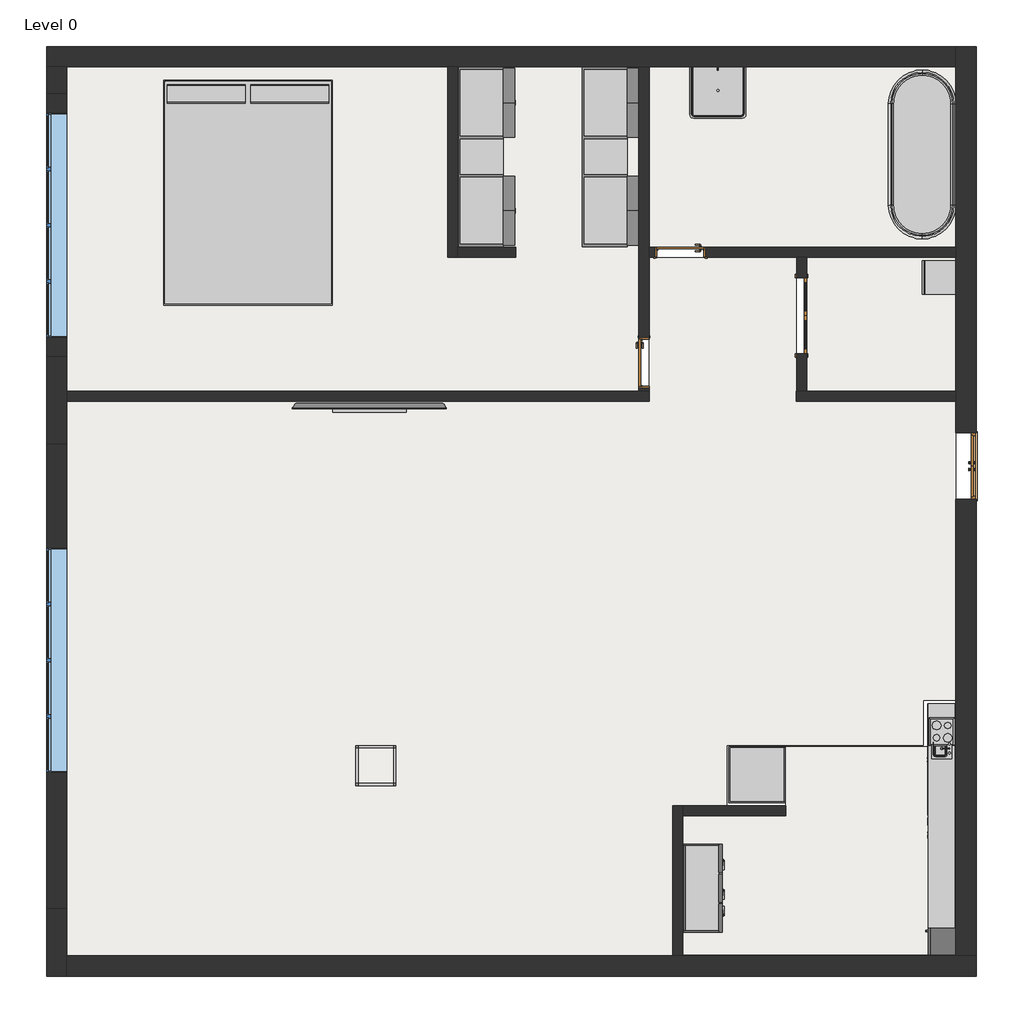
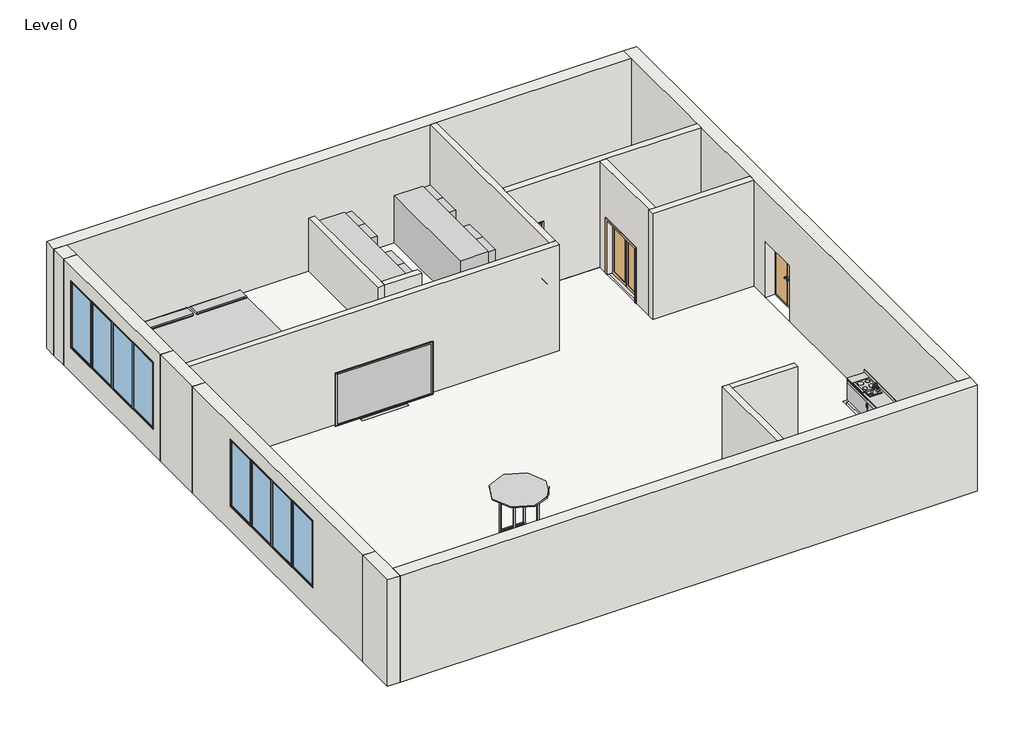
# One storey, incomplete: 17 walls, 7 furniture elements, 5 proxies, 4 doors, 4 flow terminals, 4 slabs, 2 windows.
"""IFC4 building model written with IfcOpenShell, lengths in millimetres."""

from ifc_helpers import new_model, si_unit, frame, origin, origin_with_axes, place, context, project, spatial, polyline, outline, extrude, faceted_brep, transform, mapped, element, save
from components import proxy_a6faaae8, proxy_45b28599, proxy_233f0198, kitchenette_medium_kitchenette_medium_eaec4ed0, proxy_c523a7b7, door_bbcd5f29, doors_extdbl_flush_1510x2110mm_ebd05307, doors_intsgl_1143x2413mm_ac4b68bc, flow_terminal_871c2e40, flow_terminal_6a24c7e0, flow_terminal_2cf38851, flow_terminal_2ef58978, furniture_0647d374, furniture_14b7b6c7, furniture_d6024f60, furniture_eacb8e26, furniture_d0237233, furniture_4371de90, window_3db9eff8

model = new_model("IFC4")

# Units and contexts
model_context = context("Model", 3, world=origin())
ifc_project = project(units=[si_unit("LENGTHUNIT", "METRE", prefix="MILLI")], contexts=[model_context])

# Site, building, storey
site = spatial("IfcSite", under=ifc_project)
building = spatial("IfcBuilding", under=site)
storey = spatial("IfcBuildingStorey", under=building, Name="Level 0", Elevation=0.0)

# Proxies
placement = place(None, origin())
proxy_shape = proxy_a6faaae8(model_context)
element("IfcBuildingElementProxy", 1, Name="Cook Top-4 Unit2 : 22\" x 20\"", ObjectType="Cook Top-4 Unit2 : 22\" x 20\"", at=placement, inside=storey, context=model_context, shape_type="MappedRepresentation", body=[
    mapped(proxy_shape, transform((-8192.0196087, -11110.3672005, 1.7), x_axis=(0.0, 1.0, 0.0), y_axis=(-1.0, 0.0, 0.0), z_axis=(0.0, 0.0, 1.0))),
])
proxy_2_shape = proxy_45b28599(model_context)
element("IfcBuildingElementProxy", 2, Name="Dishwasher : 24\" x 24\" x 34\"", ObjectType="Dishwasher : 24\" x 24\" x 34\"", at=placement, inside=storey, context=model_context, shape_type="MappedRepresentation", body=[
    mapped(proxy_2_shape, transform((-8452.1191735, -12937.849732, 0.0), x_axis=(0.0, -1.0, 0.0), y_axis=(1.0, 0.0, 0.0), z_axis=(0.0, 0.0, 1.0))),
])
proxy_3_shape = proxy_233f0198(model_context)
element("IfcBuildingElementProxy", 3, Name="Freezer-3 Door : 78\" x 34\"", ObjectType="Freezer-3 Door : 78\" x 34\"", at=placement, inside=storey, context=model_context, shape_type="MappedRepresentation", body=[
    mapped(proxy_3_shape, transform((-13629.6545186, -14593.5160578, 0.0), x_axis=(0.0, 1.0, 0.0), y_axis=(-1.0, 0.0, 0.0), z_axis=(0.0, 0.0, 1.0))),
])
kitchenette_medium_kitchenette_medium_shape = kitchenette_medium_kitchenette_medium_eaec4ed0(model_context)
element("IfcBuildingElementProxy", 4, Name="Kitchenette - Medium : Kitchenette - Medium", ObjectType="Kitchenette - Medium : Kitchenette - Medium", at=placement, inside=storey, context=model_context, shape_type="MappedRepresentation", body=[
    mapped(kitchenette_medium_kitchenette_medium_shape, transform((-7880.8696087, -11726.6294956, 0.0), x_axis=(0.0, -1.0, 0.0), y_axis=(1.0, 0.0, 0.0), z_axis=(0.0, 0.0, 1.0))),
])
proxy_4_shape = proxy_c523a7b7(model_context)
element("IfcBuildingElementProxy", 5, Name="Refrigerator : 24\" x 25\" LH", ObjectType="Refrigerator : 24\" x 25\" LH", at=placement, inside=storey, context=model_context, shape_type="MappedRepresentation", body=[
    mapped(proxy_4_shape, transform((-8180.5185802, -15853.8172005, 0.0), x_axis=(0.0, -1.0, 0.0), y_axis=(1.0, 0.0, 0.0), z_axis=(0.0, 0.0, 1.0))),
])

# Doors
door_shape = door_bbcd5f29(model_context)
element("IfcDoor", 6, ObjectType="Door-Double-Glass : 68\" x 80\"", at=placement, inside=storey, context=model_context, shape_type="MappedRepresentation", body=[
    mapped(door_shape, transform((-11369.4008587, -1712.3672005, 0.0), x_axis=(0.0, -1.0, 0.0), y_axis=(1.0, 0.0, 0.0), z_axis=(0.0, 0.0, 1.0))),
])
doors_extdbl_flush_1510x2110mm_shape = doors_extdbl_flush_1510x2110mm_ebd05307(model_context)
element("IfcDoor", 7, ObjectType="Doors_ExtDbl_Flush : 1510x2110mm", at=placement, inside=storey, context=model_context, shape_type="MappedRepresentation", body=[
    mapped(doors_extdbl_flush_1510x2110mm_shape, transform((-7652.2696087, -5108.9672005, 0.0), x_axis=(0.0, -1.0, 0.0), y_axis=(1.0, 0.0, 0.0), z_axis=(0.0, 0.0, 1.0))),
])
doors_intsgl_1143x2413mm_shape = doors_intsgl_1143x2413mm_ac4b68bc(model_context)
element("IfcDoor", 8, ObjectType="Doors_IntSgl : 1143x2413mm", at=placement, inside=storey, context=model_context, shape_type="MappedRepresentation", body=[
    mapped(doors_intsgl_1143x2413mm_shape, transform((-14106.8696087, -277.2672005, 0.0), x_axis=(-1.0, 0.0, 0.0), y_axis=(0.0, -1.0, 0.0), z_axis=(0.0, 0.0, 1.0))),
])
element("IfcDoor", 9, ObjectType="Doors_IntSgl : 1143x2413mm", at=placement, inside=storey, context=model_context, shape_type="MappedRepresentation", body=[
    mapped(doors_intsgl_1143x2413mm_shape, transform((-14929.3696087, -2776.1672005, 0.0), x_axis=(0.0, -1.0, 0.0), y_axis=(1.0, 0.0, 0.0), z_axis=(0.0, 0.0, 1.0))),
])

# Flow terminals
flow_terminal_shape = flow_terminal_871c2e40(model_context)
element("IfcFlowTerminal", 10, ObjectType="Sink Kitchen-Island : 18\" x 18\"", at=placement, inside=storey, context=model_context, shape_type="MappedRepresentation", body=[
    mapped(flow_terminal_shape, transform((-8200.7150099, -11475.6779599, -12.7), x_axis=(0.0, -1.0, 0.0), y_axis=(1.0, 0.0, 0.0), z_axis=(0.0, 0.0, 1.0))),
])
flow_terminal_2_shape = flow_terminal_6a24c7e0(model_context)
element("IfcFlowTerminal", 11, ObjectType="Sink Vanity-Square : 20\" x 18\"", at=placement, inside=storey, context=model_context, shape_type="MappedRepresentation", body=[
    mapped(flow_terminal_2_shape, transform((-13275.0088493, 3428.7873984, 0.0), x_axis=(1.0, 0.0, 0.0), y_axis=(0.0, 1.0, 0.0), z_axis=(0.0, 0.0, 1.0))),
])
flow_terminal_3_shape = flow_terminal_2cf38851(model_context)
element("IfcFlowTerminal", 12, ObjectType="Tub-Free Standing-3D : 30\" x 60\"", at=placement, inside=storey, context=model_context, shape_type="MappedRepresentation", body=[
    mapped(flow_terminal_3_shape, transform((-8642.8696087, 1932.5327995, 0.0), x_axis=(1.0, 0.0, 0.0), y_axis=(0.0, 1.0, 0.0), z_axis=(0.0, 0.0, 1.0))),
])
flow_terminal_4_shape = flow_terminal_2ef58978(model_context)
element("IfcFlowTerminal", 13, ObjectType="Washing Machine : 26\"x26\" - Private", at=placement, inside=storey, context=model_context, shape_type="MappedRepresentation", body=[
    mapped(flow_terminal_4_shape, transform((-8642.8696087, -848.7672005, 0.0), x_axis=(1.0, 0.0, 0.0), y_axis=(0.0, 1.0, 0.0), z_axis=(0.0, 0.0, 1.0))),
])

# Furniture
furniture_shape = furniture_0647d374(model_context)
element("IfcFurniture", 14, ObjectType="Bed-Box : Queen 60\" x 79\"", at=placement, inside=storey, context=model_context, shape_type="MappedRepresentation", body=[
    mapped(furniture_shape, transform((-24215.6720678, 1303.3623077, 0.0), x_axis=(1.0, 0.0, 0.0), y_axis=(0.0, 1.0, 0.0), z_axis=(0.0, 0.0, 1.0))),
])
furniture_2_shape = furniture_14b7b6c7(model_context)
element("IfcFurniture", 15, ObjectType="Cabinet File-Lateral 2 Drawer : 36\" x 20\" x 24\"", at=placement, inside=storey, context=model_context, shape_type="MappedRepresentation", body=[
    mapped(furniture_2_shape, transform((-13310.9879848, -11901.8946865, 0.0), x_axis=(0.0, 1.0, 0.0), y_axis=(-1.0, 0.0, 0.0), z_axis=(0.0, 0.0, 1.0))),
])
furniture_3_shape = furniture_d6024f60(model_context)
element("IfcFurniture", 16, ObjectType="Counter Top w Sink Hole : 24\" Depth", at=placement, inside=storey, context=model_context, shape_type="MappedRepresentation", body=[
    mapped(furniture_3_shape, transform((-7880.8696087, -11675.8294956, -12.7), x_axis=(0.0, -1.0, 0.0), y_axis=(1.0, 0.0, 0.0), z_axis=(0.0, 0.0, 1.0))),
])
furniture_4_shape = furniture_eacb8e26(model_context)
element("IfcFurniture", 17, ObjectType="Entertainment Center : 72\" x 72\" x 24\"", at=placement, inside=storey, context=model_context, shape_type="MappedRepresentation", body=[
    mapped(furniture_4_shape, transform((-18885.4196087, 1881.7327995, 0.0), x_axis=(0.0, 1.0, 0.0), y_axis=(-1.0, 0.0, 0.0), z_axis=(0.0, 0.0, 1.0))),
])
element("IfcFurniture", 18, ObjectType="Entertainment Center : 72\" x 72\" x 24\"", at=placement, inside=storey, context=model_context, shape_type="MappedRepresentation", body=[
    mapped(furniture_4_shape, transform((-16091.4196087, 1881.7327995, 0.0), x_axis=(0.0, 1.0, 0.0), y_axis=(-1.0, 0.0, 0.0), z_axis=(0.0, 0.0, 1.0))),
])
furniture_5_shape = furniture_d0237233(model_context)
element("IfcFurniture", 19, ObjectType="TV - Flat Screen : 50\"", at=placement, inside=storey, context=model_context, shape_type="MappedRepresentation", body=[
    mapped(furniture_5_shape, transform((-21129.3750946, -3743.7389877, 0.0), x_axis=(1.0, 0.0, 0.0), y_axis=(0.0, 1.0, 0.0), z_axis=(0.0, 0.0, 1.0))),
])
furniture_6_shape = furniture_4371de90(model_context)
element("IfcFurniture", 20, ObjectType="Table-Dining Round : 36\" Diameter", at=placement, inside=storey, context=model_context, shape_type="MappedRepresentation", body=[
    mapped(furniture_6_shape, transform((-21090.951576, -11693.838512, 0.0), x_axis=(1.0, 0.0, 0.0), y_axis=(0.0, 1.0, 0.0), z_axis=(0.0, 0.0, 1.0))),
])

# Slabs
element("IfcSlab", 21, ObjectType="Floor-Grnd-Susp_65Scr-80Ins-100Blk-75PC", at=placement, inside=storey, context=model_context, shape_type="SweptSolid", body=[
    extrude(outline(polyline([(-27972.2696087, -16177.6672005), (-27972.2696087, -3649.1172005), (-14815.0696087, -3649.1172005), (-14815.0696087, -397.9172005), (-11487.6696087, -397.9172005), (-11487.6696087, -3649.1172005), (-7880.8696087, -3649.1172005), (-7880.8696087, -10399.1672005), (-8617.4696087, -10399.1672005), (-8617.4696087, -11415.1672005), (-9404.8696087, -11415.1672005), (-13062.4696087, -11415.1672005), (-13062.4696087, -12786.7672005), (-14281.6696087, -12786.7672005), (-14281.6696087, -16177.6672005), (-27972.2696087, -16177.6672005)])), frame((0.0, 0.0, -228.6), z_axis=(0.0, 0.0, 1.0), x_axis=(1.0, 0.0, 0.0)), (0.0, 0.0, 1.0), 228.6),
])
element("IfcSlab", 22, ObjectType="Floor_Timber_22Cbd-225Joist", at=placement, inside=storey, context=model_context, shape_type="SweptSolid", body=[
    extrude(outline(polyline([(-8515.8696087, -11446.9172005), (-8515.8696087, -10481.7172005), (-7880.8696087, -10481.7172005), (-7880.8696087, -16152.2672005), (-14053.0696087, -16152.2672005), (-14053.0696087, -13015.3672005), (-11728.9696087, -13015.3672005), (-11728.9696087, -11446.9172005), (-8515.8696087, -11446.9172005)])), frame((0.0, 0.0, -228.6), z_axis=(0.0, 0.0, 1.0), x_axis=(1.0, 0.0, 0.0)), (0.0, 0.0, 1.0), 228.6),
])
element("IfcSlab", 23, ObjectType="Floor_Timber_22Cbd-225Joist", at=placement, inside=storey, context=model_context, shape_type="SweptSolid", body=[
    extrude(outline(polyline([(-14815.0696087, -162.9672005), (-14815.0696087, 3913.7327995), (-7880.8696087, 3913.7327995), (-7880.8696087, -162.9672005), (-14815.0696087, -162.9672005)])), frame((0.0, 0.0, -228.6), z_axis=(0.0, 0.0, 1.0), x_axis=(1.0, 0.0, 0.0)), (0.0, 0.0, 1.0), 228.6),
    extrude(outline(polyline([(-11252.7196087, -3420.5172005), (-11252.7196087, -391.5672005), (-7880.8696087, -391.5672005), (-7880.8696087, -3420.5172005), (-11252.7196087, -3420.5172005)])), frame((0.0, 0.0, -228.6), z_axis=(0.0, 0.0, 1.0), x_axis=(1.0, 0.0, 0.0)), (0.0, 0.0, 1.0), 228.6),
])
element("IfcSlab", 24, ObjectType="Floor_Timber_22Cbd-225Joist", at=placement, inside=storey, context=model_context, shape_type="SweptSolid", body=[
    extrude(outline(polyline([(-27972.2696087, -3420.5172005), (-27972.2696087, 3913.7327995), (-15043.6696087, 3913.7327995), (-15043.6696087, -3420.5172005), (-27972.2696087, -3420.5172005)])), frame((0.0, 0.0, -228.6), z_axis=(0.0, 0.0, 1.0), x_axis=(1.0, 0.0, 0.0)), (0.0, 0.0, 1.0), 228.6),
])

# Walls
element("IfcWall", 25, ObjectType="Wall-Ret_300Con", at=placement, inside=storey, context=model_context, shape_type="Brep", body=[
    faceted_brep([(-27972.2696087, -3649.1172005, 0.0), (-14815.0696087, -3649.1172005, 0.0), (-14815.0696087, -3649.1172005, 4000.0), (-27972.2696087, -3649.1172005, 4000.0), (-27972.2696087, -3420.5172005, 0.0), (-27972.2696087, -3420.5172005, 4000.0), (-15043.6696087, -3420.5172005, 4000.0), (-14815.0696087, -3420.5172005, 4000.0), (-14815.0696087, -3420.5172005, 0.0), (-15043.6696087, -3420.5172005, 0.0)], [[[0, 1, 2, 3]], [[4, 5, 6, 7, 8, 9]], [[1, 0, 4, 9, 8]], [[3, 2, 7, 6, 5]], [[0, 3, 5, 4]], [[2, 1, 8, 7]]]),
])
element("IfcWall", 26, ObjectType="Wall-Ret_300Con", at=placement, inside=storey, context=model_context, shape_type="Brep", body=[
    faceted_brep([(-15043.6696087, -3420.5172005, 4000.0), (-15043.6696087, 3913.7327995, 4000.0), (-15043.6696087, 3913.7327995, 0.0), (-15043.6696087, -2204.6672005, 0.0), (-15043.6696087, -2204.6672005, 2413.0), (-15043.6696087, -3347.6672005, 2413.0), (-15043.6696087, -3347.6672005, 0.0), (-15043.6696087, -3420.5172005, 0.0), (-14815.0696087, 3913.7327995, 4000.0), (-14815.0696087, -162.9672005, 4000.0), (-14815.0696087, -391.5672005, 4000.0), (-14815.0696087, -3420.5172005, 4000.0), (-14815.0696087, -3420.5172005, 0.0), (-14815.0696087, -3347.6672005, 0.0), (-14815.0696087, -3347.6672005, 2413.0), (-14815.0696087, -2204.6672005, 2413.0), (-14815.0696087, -2204.6672005, 0.0), (-14815.0696087, -391.5672005, 0.0), (-14815.0696087, -162.9672005, 0.0), (-14815.0696087, 3913.7327995, 0.0)], [[[0, 1, 2, 3, 4, 5, 6, 7]], [[8, 9, 10, 11, 12, 13, 14, 15, 16, 17, 18, 19]], [[2, 19, 18, 17, 16, 3]], [[12, 7, 6, 13]], [[1, 0, 11, 10, 9, 8]], [[2, 1, 8, 19]], [[5, 14, 13, 6]], [[15, 4, 3, 16]], [[0, 7, 12, 11]], [[4, 15, 14, 5]]]),
])
element("IfcWall", 27, ObjectType="Wall-Ret_300Con", at=placement, inside=storey, context=model_context, shape_type="Brep", body=[
    faceted_brep([(-7880.8696087, -391.5672005, 4000.0), (-11252.7196087, -391.5672005, 4000.0), (-11481.3196087, -391.5672005, 4000.0), (-14815.0696087, -391.5672005, 4000.0), (-14815.0696087, -391.5672005, 0.0), (-14678.3696087, -391.5672005, 0.0), (-14678.3696087, -391.5672005, 2413.0), (-13535.3696087, -391.5672005, 2413.0), (-13535.3696087, -391.5672005, 0.0), (-11481.3196087, -391.5672005, 0.0), (-11252.7196087, -391.5672005, 0.0), (-7880.8696087, -391.5672005, 0.0), (-14815.0696087, -162.9672005, 4000.0), (-7880.8696087, -162.9672005, 4000.0), (-7880.8696087, -162.9672005, 0.0), (-13535.3696087, -162.9672005, 0.0), (-13535.3696087, -162.9672005, 2413.0), (-14678.3696087, -162.9672005, 2413.0), (-14678.3696087, -162.9672005, 0.0), (-14815.0696087, -162.9672005, 0.0)], [[[0, 1, 2, 3, 4, 5, 6, 7, 8, 9, 10, 11]], [[12, 13, 14, 15, 16, 17, 18, 19]], [[4, 19, 18, 5]], [[14, 11, 10, 9, 8, 15]], [[3, 2, 1, 0, 13, 12]], [[0, 11, 14, 13]], [[4, 3, 12, 19]], [[17, 6, 5, 18]], [[7, 16, 15, 8]], [[16, 7, 6, 17]]]),
])
element("IfcWall", 28, ObjectType="Wall-Ret_300Con", at=placement, inside=storey, context=model_context, shape_type="SweptSolid", body=[
    extrude(outline(polyline([(-3420.5172005, 4000.0), (-391.5672005, 4000.0), (-391.5672005, 0.0), (-848.7672005, 0.0), (-848.7672005, 2032.0), (-2575.9672005, 2032.0), (-2575.9672005, 0.0), (-3420.5172005, 0.0), (-3420.5172005, 4000.0)])), frame((-11481.3196087, 0.0, 0.0), z_axis=(1.0, 0.0, 0.0), x_axis=(0.0, 1.0, 0.0)), (0.0, 0.0, 1.0), 228.6),
])
element("IfcWall", 29, ObjectType="Wall-Ret_300Con", at=placement, inside=storey, context=model_context, shape_type="Brep", body=[
    faceted_brep([(-14053.0696087, -16177.6672005, 0.0), (-14053.0696087, -13015.3672005, 0.0), (-14053.0696087, -12786.7672005, 0.0), (-14053.0696087, -12786.7672005, 4000.0), (-14053.0696087, -13015.3672005, 4000.0), (-14053.0696087, -16177.6672005, 4000.0), (-14281.6696087, -16177.6672005, 0.0), (-14281.6696087, -16177.6672005, 4000.0), (-14281.6696087, -12786.7672005, 4000.0), (-14281.6696087, -12786.7672005, 0.0)], [[[0, 1, 2, 3, 4, 5]], [[6, 7, 8, 9]], [[2, 1, 0, 6, 9]], [[5, 4, 3, 8, 7]], [[0, 5, 7, 6]], [[3, 2, 9, 8]]]),
])
element("IfcWall", 30, ObjectType="Wall-Ret_300Con", at=placement, inside=storey, context=model_context, shape_type="SweptSolid", body=[
    extrude(outline(polyline([(-11728.9696087, -13015.3672005), (-14053.0696087, -13015.3672005), (-14053.0696087, -12786.7672005), (-11728.9696087, -12786.7672005), (-11728.9696087, -13015.3672005)])), origin_with_axes(), (0.0, 0.0, 1.0), 4000.0),
])
element("IfcWall", 31, ObjectType="Wall-Ret_300Con", at=placement, inside=storey, context=model_context, shape_type="Brep", body=[
    faceted_brep([(-19368.0196087, 3913.7327995, 0.0), (-19368.0196087, -391.5672005, 0.0), (-19368.0196087, -391.5672005, 2000.0), (-19368.0196087, 3913.7327995, 2000.0), (-19139.4196087, 3913.7327995, 0.0), (-19139.4196087, 3913.7327995, 2000.0), (-19139.4196087, -162.9672005, 2000.0), (-19139.4196087, -391.5672005, 2000.0), (-19139.4196087, -391.5672005, 0.0), (-19139.4196087, -162.9672005, 0.0)], [[[0, 1, 2, 3]], [[4, 5, 6, 7, 8, 9]], [[1, 0, 4, 9, 8]], [[3, 2, 7, 6, 5]], [[0, 3, 5, 4]], [[2, 1, 8, 7]]]),
])
element("IfcWall", 32, ObjectType="Wall-Ret_300Con", at=placement, inside=storey, context=model_context, shape_type="SweptSolid", body=[
    extrude(outline(polyline([(-17831.3196087, -391.5672005), (-19139.4196087, -391.5672005), (-19139.4196087, -162.9672005), (-17831.3196087, -162.9672005), (-17831.3196087, -391.5672005)])), origin_with_axes(), (0.0, 0.0, 1.0), 2000.0),
])
element("IfcWall", 33, ObjectType="Wall-Ret_300Con", at=placement, inside=storey, context=model_context, shape_type="Brep", body=[
    faceted_brep([(-11487.6696087, -3649.1172005, 0.0), (-7880.8696087, -3649.1172005, 0.0), (-7880.8696087, -3649.1172005, 4000.0), (-11487.6696087, -3649.1172005, 4000.0), (-11487.6696087, -3420.5172005, 0.0), (-11487.6696087, -3420.5172005, 4000.0), (-11481.3196087, -3420.5172005, 4000.0), (-11252.7196087, -3420.5172005, 4000.0), (-7880.8696087, -3420.5172005, 4000.0), (-7880.8696087, -3420.5172005, 0.0), (-11252.7196087, -3420.5172005, 0.0), (-11481.3196087, -3420.5172005, 0.0)], [[[0, 1, 2, 3]], [[4, 5, 6, 7, 8, 9, 10, 11]], [[1, 0, 4, 11, 10, 9]], [[3, 2, 8, 7, 6, 5]], [[0, 3, 5, 4]], [[2, 1, 9, 8]]]),
])
element("IfcWall", 34, ObjectType="Wall-Ret_300Con 3", at=placement, inside=storey, context=model_context, shape_type="Brep", body=[
    faceted_brep([(-28429.4696087, 3913.7327995, 0.0), (-27972.2696087, 3913.7327995, 0.0), (-19368.0196087, 3913.7327995, 0.0), (-19139.4196087, 3913.7327995, 0.0), (-15043.6696087, 3913.7327995, 0.0), (-14815.0696087, 3913.7327995, 0.0), (-7880.8696087, 3913.7327995, 0.0), (-7880.8696087, 3913.7327995, 4000.0), (-14815.0696087, 3913.7327995, 4000.0), (-15043.6696087, 3913.7327995, 4000.0), (-27972.2696087, 3913.7327995, 4000.0), (-28429.4696087, 3913.7327995, 4000.0), (-28429.4696087, 4370.9327995, 0.0), (-28429.4696087, 4370.9327995, 4000.0), (-7880.8696087, 4370.9327995, 4000.0), (-7880.8696087, 4370.9327995, 0.0)], [[[0, 1, 2, 3, 4, 5, 6, 7, 8, 9, 10, 11]], [[12, 13, 14, 15]], [[6, 5, 4, 3, 2, 1, 0, 12, 15]], [[11, 10, 9, 8, 7, 14, 13]], [[0, 11, 13, 12]], [[7, 6, 15, 14]]]),
])
element("IfcWall", 35, ObjectType="Wall-Ret_300Con 3", at=placement, inside=storey, context=model_context, shape_type="Brep", body=[
    faceted_brep([(-27972.2696087, -16634.8672005, 0.0), (-27972.2696087, -16177.6672005, 0.0), (-27972.2696087, -15110.8672005, 0.0), (-27972.2696087, -15110.8672005, 4000.0), (-27972.2696087, -16177.6672005, 4000.0), (-27972.2696087, -16634.8672005, 4000.0), (-28429.4696087, -16634.8672005, 0.0), (-28429.4696087, -16634.8672005, 4000.0), (-28429.4696087, -15110.8672005, 4000.0), (-28429.4696087, -15110.8672005, 0.0)], [[[0, 1, 2, 3, 4, 5]], [[6, 7, 8, 9]], [[2, 1, 0, 6, 9]], [[3, 2, 9, 8]], [[5, 4, 3, 8, 7]], [[0, 5, 7, 6]]]),
])
element("IfcWall", 36, ObjectType="Wall-Ret_300Con 3", at=placement, inside=storey, context=model_context, shape_type="Brep", body=[
    faceted_brep([(-7423.6696087, -16177.6672005, 0.0), (-7880.8696087, -16177.6672005, 0.0), (-14053.0696087, -16177.6672005, 0.0), (-14281.6696087, -16177.6672005, 0.0), (-27972.2696087, -16177.6672005, 0.0), (-27972.2696087, -16177.6672005, 4000.0), (-14281.6696087, -16177.6672005, 4000.0), (-14053.0696087, -16177.6672005, 4000.0), (-7880.8696087, -16177.6672005, 4000.0), (-7423.6696087, -16177.6672005, 4000.0), (-7423.6696087, -16634.8672005, 0.0), (-7423.6696087, -16634.8672005, 4000.0), (-27972.2696087, -16634.8672005, 4000.0), (-27972.2696087, -16634.8672005, 0.0)], [[[0, 1, 2, 3, 4, 5, 6, 7, 8, 9]], [[10, 11, 12, 13]], [[4, 3, 2, 1, 0, 10, 13]], [[9, 8, 7, 6, 5, 12, 11]], [[0, 9, 11, 10]], [[5, 4, 13, 12]]]),
])
element("IfcWall", 37, ObjectType="Wall-Ret_300Con 3", at=placement, inside=storey, context=model_context, shape_type="Brep", body=[
    faceted_brep([(-7880.8696087, -16177.6672005, 4000.0), (-7880.8696087, -3649.1172005, 4000.0), (-7880.8696087, -3420.5172005, 4000.0), (-7880.8696087, -391.5672005, 4000.0), (-7880.8696087, -162.9672005, 4000.0), (-7880.8696087, 3913.7327995, 4000.0), (-7880.8696087, 4370.9327995, 4000.0), (-7880.8696087, 4370.9327995, 0.0), (-7880.8696087, 3913.7327995, 0.0), (-7880.8696087, -162.9672005, 0.0), (-7880.8696087, -391.5672005, 0.0), (-7880.8696087, -3420.5172005, 0.0), (-7880.8696087, -3649.1172005, 0.0), (-7880.8696087, -4353.9672005, 0.0), (-7880.8696087, -4353.9672005, 2110.0), (-7880.8696087, -5863.9672005, 2110.0), (-7880.8696087, -5863.9672005, 0.0), (-7880.8696087, -16177.6672005, 0.0), (-7423.6696087, 4370.9327995, 4000.0), (-7423.6696087, -16177.6672005, 4000.0), (-7423.6696087, -16177.6672005, 0.0), (-7423.6696087, -5863.9672005, 0.0), (-7423.6696087, -5863.9672005, 2110.0), (-7423.6696087, -4353.9672005, 2110.0), (-7423.6696087, -4353.9672005, 0.0), (-7423.6696087, 4370.9327995, 0.0)], [[[0, 1, 2, 3, 4, 5, 6, 7, 8, 9, 10, 11, 12, 13, 14, 15, 16, 17]], [[18, 19, 20, 21, 22, 23, 24, 25]], [[7, 25, 24, 13, 12, 11, 10, 9, 8]], [[20, 17, 16, 21]], [[6, 5, 4, 3, 2, 1, 0, 19, 18]], [[7, 6, 18, 25]], [[0, 17, 20, 19]], [[23, 14, 13, 24]], [[15, 22, 21, 16]], [[14, 23, 22, 15]]]),
])
element("IfcWall", 38, ObjectType="Wall-Ret_300Con 3", at=placement, inside=storey, context=model_context, shape_type="SweptSolid", body=[
    extrude(outline(polyline([(-27972.2696087, 3913.7327995), (-27972.2696087, 3304.1327995), (-28429.4696087, 3304.1327995), (-28429.4696087, 3913.7327995), (-27972.2696087, 3913.7327995)])), origin_with_axes(), (0.0, 0.0, 1.0), 4000.0),
])
element("IfcWall", 39, ObjectType="Wall-Ret_300Con 3", at=placement, inside=storey, context=model_context, shape_type="Brep", body=[
    faceted_brep([(-27972.2696087, -4620.6672005, 0.0), (-27972.2696087, -3649.1172005, 0.0), (-27972.2696087, -3420.5172005, 0.0), (-27972.2696087, -2639.4672005, 0.0), (-27972.2696087, -2639.4672005, 4000.0), (-27972.2696087, -3420.5172005, 4000.0), (-27972.2696087, -3649.1172005, 4000.0), (-27972.2696087, -4620.6672005, 4000.0), (-28429.4696087, -4620.6672005, 0.0), (-28429.4696087, -4620.6672005, 4000.0), (-28429.4696087, -2639.4672005, 4000.0), (-28429.4696087, -2639.4672005, 0.0)], [[[0, 1, 2, 3, 4, 5, 6, 7]], [[8, 9, 10, 11]], [[3, 2, 1, 0, 8, 11]], [[4, 3, 11, 10]], [[7, 6, 5, 4, 10, 9]], [[0, 7, 9, 8]]]),
])
element("IfcWall", 40, ObjectType="Wall-Ret_300Con 3", at=placement, inside=storey, context=model_context, shape_type="SweptSolid", body=[
    extrude(outline(polyline([(3304.1327995, 0.0), (-2639.4672005, 0.0), (-2639.4672005, 4000.0), (3304.1327995, 4000.0), (3304.1327995, 0.0)]), holes=[polyline([(2872.3327995, 914.4), (2872.3327995, 3454.4), (-2207.6672005, 3454.4), (-2207.6672005, 914.4), (2872.3327995, 914.4)])]), frame((-28429.4696087, 0.0, 0.0), z_axis=(1.0, 0.0, 0.0), x_axis=(0.0, 1.0, 0.0)), (0.0, 0.0, 1.0), 457.2),
])
element("IfcWall", 41, ObjectType="Wall-Ret_300Con 3", at=placement, inside=storey, context=model_context, shape_type="SweptSolid", body=[
    extrude(outline(polyline([(-4620.6672005, 0.0), (-15110.8672005, 0.0), (-15110.8672005, 4000.0), (-4620.6672005, 4000.0), (-4620.6672005, 0.0)]), holes=[polyline([(-6957.4672005, 914.4), (-6957.4672005, 3454.4), (-12037.4672005, 3454.4), (-12037.4672005, 914.4), (-6957.4672005, 914.4)])]), frame((-28429.4696087, 0.0, 0.0), z_axis=(1.0, 0.0, 0.0), x_axis=(0.0, 1.0, 0.0)), (0.0, 0.0, 1.0), 457.2),
])

# Windows
window_shape = window_3db9eff8(model_context)
element("IfcWindow", 42, ObjectType="Window-Casement-Multi-Sash-Horizontal : 200\" x 100\"", at=placement, inside=storey, context=model_context, shape_type="MappedRepresentation", body=[
    mapped(window_shape, transform((-28200.8696087, -9497.4672005, 0.0), x_axis=(0.0, 1.0, 0.0), y_axis=(-1.0, 0.0, 0.0), z_axis=(0.0, 0.0, 1.0))),
])
element("IfcWindow", 43, ObjectType="Window-Casement-Multi-Sash-Horizontal : 200\" x 100\"", at=placement, inside=storey, context=model_context, shape_type="MappedRepresentation", body=[
    mapped(window_shape, transform((-28200.8696087, 332.3327995, 0.0), x_axis=(0.0, 1.0, 0.0), y_axis=(-1.0, 0.0, 0.0), z_axis=(0.0, 0.0, 1.0))),
])

save(model, "model.ifc")

# Revit data of these elements
# Type "Cook Top-4 Unit2 : 22\" x 20\""
#   Depth = 1' - 8"
#   Width = 1' - 10"
#   Burner Material = Steel, Chrome Plated
#   Cooktop Material = Steel, Polished
#   Default Elevation = 0
#   Assembly Code = ""
# Type "Dishwasher : 24\" x 24\" x 34\""
#   Label = "DW"
#   Assembly Code = "E1090400"
#   Depth = 2' - 0"
#   Height = 2' - 10"
#   Width = 2' - 0"
#   Dishwasher Material = Steel, Paint Finish, Ivory, Glossy
#   Panel Face Material = Plastic, Opaque Black
#   Default Elevation = 0
# Type "Freezer-3 Door : 78\" x 34\""
#   Assembly Code = "E1090320"
#   Description = "Reach-In Freezer"
#   Depth = 2' - 10"
#   Height = 6' - 7 1/4"
#   Width = 6' - 6"
#   Default Elevation = 0
# Type "Kitchenette - Medium : Kitchenette - Medium"
#   Assembly Code = "E1090400"
#   Sink Opening Depth = 1' - 2"
#   Sink Location To Wall = 0' - 6"
#   Sink Location = 3' - 4"
#   Counter Thickness = 0' - 1 1/2"
#   Counter Length = 16' - 8"
#   Cabinet Width = 8' - 4"
#   Cabinet Height = 2' - 10"
#   Cabinet Depth = 2' - 0 1/2"
#   Toe Depth = 0' - 3"
#   Toe Height = 0' - 3 1/2"
#   Cabinet Material = Cabinets
#   Door/Drawer Material = Cabinets
#   Handle Material = Cabinets - Handles
#   Default Elevation = 0
# Type "Refrigerator : 24\" x 25\" LH"
#   Label = "REF."
#   Assembly Code = "E1090400"
#   Depth = 2' - 0 3/4"
#   Handle = 0' - 1 1/2"
#   Height = 5' - 3 1/2"
#   Rear Clearance = 0' - 2"
#   Top Door Height = 1' - 8"
#   Width = 1' - 11 1/2"
#   Material = Steel, Paint Finish, Ivory, Glossy
#   Default Elevation = 0
# Type "Door-Double-Glass : 68\" x 80\""
#   Type Mark = "46"
#   Construction Type Id = "opn-d45"
#   Assembly Code = "C1020"
#   Analytic Construction = "Wood frame, double glass door "
#   W = 2' - 10"
#   Thickness = 0' - 2"
#   Thermal Resistance (R) = 0.31964 (m²·K)/W
#   Swing Angle [instance default] = 90.00°
#   Heat Transfer Coefficient (U) = 3.12872 W/(m²·K)
#   Height = 6' - 8"
#   Bottom Rail = 0' - 4"
#   Top Rail = 0' - 4"
#   Stiles = 0' - 4"
#   Trim Projection = 0' - 1"
#   Trim Width = 0' - 3"
#   Width = 5' - 8"
#   Define Thermal Properties by = 1
#   Glazing = Glass
#   Panel Material = Wood - Birch - Solid Stained Light Low Gloss
#   Trim Material = Paint - Sienna
#   Visual Light Transmittance = 0
#   Solar Heat Gain Coefficient = 0
#   Function = (empty or 0)
#   Wall Closure = (empty or 0)
# Type "Doors_ExtDbl_Flush : 1510x2110mm"
#   Construction Type Id = "MDOOR"
#   Type Mark = "45"
#   Type Comments = "External Double"
#   Operation = "DoubleDoorSingleSwing"
#   Keynote = "L20"
#   Analytic Construction = "Metal"
#   Wrap Layers (Ext) from Ext = 0' - 4.03543"
#   Wrap Layers (Int) from Ext = 0' - 6.98819"
#   Thickness = 0' - 1.73228"
#   Rough Width = 4' - 11.44882"
#   Rough Height = 6' - 11.07087"
#   O/A Frame Width = 0' - 2.51969"
#   Heat Transfer Coefficient (U) = 3.7021 W/(m²·K)
#   Handle Z Distance = 3' - 5.33858"
#   FrameWidth = 0' - 1.65354"
#   FrameOffset - External = 0' - 0.98425"
#   FrameDepth = 0' - 3.50394"
#   Door Panel Width = 2' - 3.6378"
#   Door Panel Thickness = 0' - 1.73228"
#   Door Panel Height = 6' - 6.74016"
#   Cill Thickness = 0' - 2.14567"
#   Cill Projection = 0' - 1.1811"
#   Handle X Distance = 0' - 2.95276"
#   Height = 6' - 11.07087"
#   Structural Tolerance = 0' - 0.25591"
#   Tolerance = 0' - 0.11811"
#   Undercut = 0' - 0.15748"
#   Width = 4' - 11.44882"
#   Cill Extension = 0' - 0.98425"
#   Cavity Closer Width = 0' - 1.9685"
#   Cavity Closer Offset from Ext = 0' - 4.03543"
#   Cavity Closer Depth = 0' - 3.34646"
#   Define Thermal Properties by = 1
#   Vis - Ironmongery = yes
#   Vis - Cavity Closers = yes
#   Function = 1
#   Material Door = Door - Panel
#   Material Frame = Door - Frame/Mullion
#   Material Ironmongery = Door - Handle
#   Visual Light Transmittance = 0
#   Thermal Resistance (R) = 0
#   Solar Heat Gain Coefficient = 0
#   Wall Closure = (empty or 0)
# Type "Doors_IntSgl : 1143x2413mm"
#   Construction Type Id = "MDOOR"
#   Type Mark = "43"
#   Type Comments = "Internal Single"
#   Operation = "SingleSwingRight"
#   Manufacturer = "Revit"
#   Keynote = "L20"
#   Description = "Internal Single Door"
#   Analytic Construction = "Metal"
#   UnderCut = 0' - 0.31496"
#   Tolerance = 0' - 0.07874"
#   Thickness = 0' - 1.49606"
#   Thermal Resistance (R) = 0.270117 (m²·K)/W
#   Structural Tolerance = 0' - 0.31496"
#   StopDepth = 0' - 1.25984"
#   Stop Thickness = 0' - 0.74803"
#   Rough Width = 3' - 9"
#   Rough Height = 7' - 11"
#   Height to Top Lock Rail = 3' - 3.37008"
#   Heat Transfer Coefficient (U) = 3.7021 W/(m²·K)
#   Handle Z Distance = 2' - 11.43307"
#   Handle X Distance = 0' - 2.95276"
#   Frame Thickness = 0' - 1.25984"
#   Door Panel Width = 3' - 5.69291"
#   Door Panel Thickness = 0' - 1.49606"
#   Door Panel Offset = 0' - 0"
#   Height = 7' - 11"
#   Width = 3' - 9"
#   Door Panel Height = 7' - 9.0315"
#   Architrave Setback = 0' - 0.19685"
#   Define Thermal Properties by = 1
#   Vis - Ironmongery = yes
#   Material Ironmongery = Door - Handle
#   Material Frame = Door - Frame/Mullion (1)
#   Material Door = Door - Panel
#   Material Architrave = Door - Architrave
#   Visual Light Transmittance = 0
#   Solar Heat Gain Coefficient = 0
#   Function = (empty or 0)
#   Wall Closure = (empty or 0)
# Type "Sink Kitchen-Island : 18\" x 18\""
#   Assembly Code = "D2010410"
#   Counter Height = 3' - 0"
#   Depth = 1' - 6"
#   Width = 1' - 6"
#   Faucet Material = Steel, Polished
#   Sink Material = Steel, Polished
#   Default Elevation = 0
# Type "Sink Vanity-Square : 20\" x 18\""
#   Assembly Code = "D2010400"
#   Counter Height = 2' - 7"
#   Depth = 4' - 2"
#   Width = 4' - 2"
#   Basin Material = Porcelain, Linen
#   Faucet Material = Steel, Polished
#   Default Elevation = 0
# Type "Tub-Free Standing-3D : 30\" x 60\""
#   Assembly Code = "D2010110"
#   Height = 1' - 6"
#   Length = 12' - 6"
#   Width = 5' - 0"
#   Tub Material = Porcelain, Ivory
#   Default Elevation = 0
# Type "Washing Machine : 26\"x26\" - Private"
#   Sanitary Radius = 25.4 mm
#   Sanitary Diameter = 50.8 mm
#   Washing Machine Width = 2' - 6"
#   Washing Machine Length = 2' - 6"
#   Washing Machine Height = 3' - 4"
#   WFU = 2
#   Voltage = 120 V
#   Hot Water Radius = 12.7 mm
#   Hot Water Diameter = 25.4 mm
#   Half Washing Machine Width = 1' - 3"
#   HWFU = 1
#   Flow Pressure [instance default] = 55158.1 Pa
#   Cold Water Radius = 12.7 mm
#   Cold Water Diameter = 25.4 mm
#   CWFU = 1
#   Apparent Load = 600 VA
#   Number of Poles = 1
#   Washing Machine Material = none
#   Default Elevation = 0
#   Assembly Code = ""
# Type "Bed-Box : Queen 60\" x 79\""
#   Assembly Code = "E2020200"
#   Length = 16' - 8"
#   Width = 12' - 6"
#   Frame Material = Copper
#   Mattress Material = Linen, White
#   Default Elevation = 0
# Type "Cabinet File-Lateral 2 Drawer : 36\" x 20\" x 24\""
#   Assembly Code = "E2020200"
#   Depth = 4' - 2"
#   Height = 6' - 3"
#   Width = 4' - 2"
#   Material = Metal - Steel
#   Default Elevation = 0
# Type "Counter Top w Sink Hole : 24\" Depth"
#   Assembly Code = "C1030400"
#   Counter Thickness = 0' - 1 1/2"
#   Depth [instance default] = 2' - 1"
#   Height = 3' - 0"
#   Length [instance default] = 8' - 0"
#   Sink Location [instance default] = 2' - 0"
#   Sink Location To Wall [instance default] = 0' - 6"
#   Sink Opening Depth [instance default] = 1' - 3"
#   Sink Opening Width [instance default] = 2' - 3"
#   Counter Top Material = none
#   Default Elevation = 0
# Type "Entertainment Center : 72\" x 72\" x 24\""
#   Assembly Code = "E2020200"
#   Center Width = 2' - 8"
#   Depth = 4' - 2"
#   Height = 5' - 10"
#   Width = 13' - 4"
#   Material = none
#   Default Elevation = 0
# Type "TV - Flat Screen : 50\""
#   SinAng = 0' - 0.0193"
#   L = 10' - 10.73345"
#   H = 6' - 1.54431"
#   Thickness = 0' - 4.33071"
#   Diagonal = 12' - 6"
#   CosAng = 0' - 0.03431"
#   Stand [instance default] = yes
#   Default Elevation = 0
# Type "Table-Dining Round : 36\" Diameter"
#   Assembly Code = "E2020200"
#   Diameter = 6' - 3"
#   Height = 6' - 3"
#   Base Material = Pine
#   Top Material = Laminate, Linen, Matte
#   Default Elevation = 0
# Type "Floor-Grnd-Susp_65Scr-80Ins-100Blk-75PC"
#   Keynote = "E60/130"
#   Function = 0
#   Layers, outside or top first: 0' - 9" "Concrete, Precast" (function 1)
# Type "Floor_Timber_22Cbd-225Joist"
#   Function = 0
#   Layers, outside or top first: 0' - 9" "Structure, Timber Joist/Rafter Layer" (function 1)
# Type "Wall-Ret_300Con"
#   Layers, outside or top first: 0' - 9" "Concrete, Cast In Situ" (function 1)
# Type "Wall-Ret_300Con 3"
#   Layers, outside or top first: 1' - 6" "Concrete, Cast In Situ" (function 1)
# Type "Window-Casement-Multi-Sash-Horizontal : 200\" x 100\""
#   Type Mark = "50"
#   Fire Rating = "0.5h"
#   Assembly Code = "B2020100"
#   Analytic Construction = "Double glazing - domestic"
#   Window Inset [instance default] = 0' - 0 5/8"
#   Wall Thickness [instance default] = 0' - 6"
#   Visual Light Transmittance = 0.81
#   Thermal Resistance (R) = 0.319569 (m²·K)/W
#   Solar Heat Gain Coefficient = 0.76
#   Rough Width = 16' - 8 1/2"
#   Rough Height = 8' - 4 1/2"
#   Open Window Width = 4' - 2"
#   Heat Transfer Coefficient (U) = 3.12929 W/(m²·K)
#   Height = 8' - 4"
#   Frame Gap 3 [instance default] = 0' - 1 83/128"
#   Frame Gap 2 [instance default] = 0' - 0 5/8"
#   Frame Gap 1 = 0' - 1 51/128"
#   Default Sill Height = 3' - 0"
#   Width = 16' - 8"
#   Frame Material = Metal - Aluminum
#   Glass Panel Material = Glass
#   Wall Closure = (empty or 0)
# Element 1 (IfcBuildingElementProxy, "Cook Top-4 Unit2 : 22\" x 20\"")
#   Phase Created = New Construction
#   Materials on its faces: "Steel, Chrome Plated", "Steel, Polished"
# Element 2 (IfcBuildingElementProxy, "Dishwasher : 24\" x 24\" x 34\"")
#   Phase Created = New Construction
#   Materials on its faces: "Steel, Paint Finish, Ivory, Glossy", "Plastic, Opaque Black"
# Element 3 (IfcBuildingElementProxy, "Freezer-3 Door : 78\" x 34\"")
#   Phase Created = New Construction
#   Materials on its faces: "Metal - Stainless Steel", "Slate"
# Element 4 (IfcBuildingElementProxy, "Kitchenette - Medium : Kitchenette - Medium")
#   Phase Created = New Construction
#   Materials on its faces: "Cabinets", "Cabinets - Handles"
# Element 5 (IfcBuildingElementProxy, "Refrigerator : 24\" x 25\" LH")
#   Phase Created = New Construction
#   Materials on its faces: "Steel, Paint Finish, Ivory, Glossy", "Steel, Chrome Plated"
# Element 6 (IfcDoor, "Door-Double-Glass : 68\" x 80\"")
#   Swing Angle = 90.00°
#   Phase Created = New Construction
#   Materials on its faces: "Wood - Birch - Solid Stained Light Low Gloss", "Paint - Sienna", "Glass"
# Element 7 (IfcDoor, "Doors_ExtDbl_Flush : 1510x2110mm")
#   Phase Created = New Construction
#   Materials on its faces: "Door - Handle", "Door - Frame/Mullion", "Door - Panel"
# Elements 8, 9 (IfcDoor, "Doors_IntSgl : 1143x2413mm")
#   Phase Created = New Construction
#   Materials on its faces: "Door - Architrave", "Door - Handle", "Door - Frame/Mullion (1)", "Door - Panel"
# Element 10 (IfcFlowTerminal, "Sink Kitchen-Island : 18\" x 18\"")
#   Mark = "1"
#   Phase Created = New Construction
#   Materials on its faces: "Steel, Polished"
# Element 11 (IfcFlowTerminal, "Sink Vanity-Square : 20\" x 18\"")
#   Mark = "4"
#   Phase Created = New Construction
#   Materials on its faces: "Porcelain, Linen", "Steel, Polished"
# Element 12 (IfcFlowTerminal, "Tub-Free Standing-3D : 30\" x 60\"")
#   Mark = "2"
#   Phase Created = New Construction
#   Materials on its faces: "Porcelain, Ivory"
# Element 13 (IfcFlowTerminal, "Washing Machine : 26\"x26\" - Private")
#   Mark = "5"
#   Flow Pressure = 55158.1 Pa
#   Phase Created = New Construction
# Element 14 (IfcFurniture, "Bed-Box : Queen 60\" x 79\"")
#   Phase Created = New Construction
#   Materials on its faces: "Copper", "Linen, White"
# Element 15 (IfcFurniture, "Cabinet File-Lateral 2 Drawer : 36\" x 20\" x 24\"")
#   Phase Created = New Construction
#   Materials on its faces: "Metal - Steel"
# Element 16 (IfcFurniture, "Counter Top w Sink Hole : 24\" Depth")
#   Sink Opening Depth = 1' - 2"
#   Sink Location To Wall = 0' - 6"
#   Length = 16' - 8"
#   Sink Location = 3' - 4"
#   Sink Opening Width = 1' - 4"
#   Depth = 2' - 0 1/2"
#   Phase Created = New Construction
#   Materials on its faces: "Counter Top"
# Elements 17, 18 (IfcFurniture, "Entertainment Center : 72\" x 72\" x 24\"")
#   Phase Created = New Construction
#   Materials on its faces: "Steel, Chrome Plated", "Glass - Clear, Grey"
# Element 19 (IfcFurniture, "TV - Flat Screen : 50\"")
#   Stand = yes
#   Phase Created = New Construction
#   Materials on its faces: "TV - Black", "TV - Glass", "TV - Screen"
# Element 20 (IfcFurniture, "Table-Dining Round : 36\" Diameter")
#   Phase Created = New Construction
#   Materials on its faces: "Pine", "Laminate, Linen, Matte"
# Element 21 (IfcSlab, "Floor-Grnd-Susp_65Scr-80Ins-100Blk-75PC")
#   built-in parameter 1001955 = -1.5708 (stored number, unit not read)
#   Height Offset From Level = 0' - 0"
#   Phase Created = New Construction
#   Materials on its faces: "Concrete, Precast"
# Element 22 (IfcSlab, "Floor_Timber_22Cbd-225Joist")
#   Height Offset From Level = 0' - 0"
#   Phase Created = New Construction
#   Materials on its faces: "Structure, Timber Joist/Rafter Layer"
# Elements 23, 24 (IfcSlab, "Floor_Timber_22Cbd-225Joist")
#   built-in parameter 1001955 = -1.5708 (stored number, unit not read)
#   Height Offset From Level = 0' - 0"
#   Phase Created = New Construction
#   Materials on its faces: "Structure, Timber Joist/Rafter Layer"
# Elements 25, 26, 27, 28, 29, 30, 33 (IfcWall, "Wall-Ret_300Con")
#   Top Offset = 0' - 0"
#   Base Offset = 0' - 0"
#   wall height = 13' - 1.48031"
#   Phase Created = New Construction
#   Base Constraint = Level 0
#   Top Constraint = Level 1
#   Materials on its faces: "Concrete, Cast In Situ"
# Elements 31, 32 (IfcWall, "Wall-Ret_300Con")
#   Top Offset = 0' - 0"
#   Base Offset = 0' - 0"
#   Unconnected Height = 6' - 6.74016"
#   wall height = 6' - 6.74016"
#   Phase Created = New Construction
#   Base Constraint = Level 0
#   Materials on its faces: "Concrete, Cast In Situ"
# Elements 34, 35, 36, 37, 38, 39, 40, 41 (IfcWall, "Wall-Ret_300Con 3")
#   Top Offset = 0' - 0"
#   Base Offset = 0' - 0"
#   wall height = 13' - 1.48031"
#   Phase Created = New Construction
#   Base Constraint = Level 0
#   Top Constraint = Level 1
#   Materials on its faces: "Concrete, Cast In Situ"
# Element 42 (IfcWindow, "Window-Casement-Multi-Sash-Horizontal : 200\" x 100\"")
#   Mark = "1"
#   Window Inset = 0' - 0 5/8"
#   Frame Gap 3 = 0' - 1 83/128"
#   Frame Gap 2 = 0' - 0 5/8"
#   Phase Created = New Construction
#   Materials on its faces: "Metal - Aluminum", "Glass"
# Element 43 (IfcWindow, "Window-Casement-Multi-Sash-Horizontal : 200\" x 100\"")
#   Mark = "2"
#   Window Inset = 0' - 0 5/8"
#   Frame Gap 3 = 0' - 1 83/128"
#   Frame Gap 2 = 0' - 0 5/8"
#   Phase Created = New Construction
#   Materials on its faces: "Metal - Aluminum", "Glass"
# Materials
#   "Steel, Chrome Plated": class "Metal", colour RGB 216 216 216, transparency 0, Description = "Chromiuim plated steel", Cost = 0
#   "Steel, Polished": class "Metal", colour RGB 57 57 57, transparency 0, Description = "Polished steel", Cost = 0
#   "Steel, Paint Finish, Ivory, Glossy": class "Metal", colour RGB 247 247 239, transparency 0, Description = "Steel, paint finish, ivory, glossy", Cost = 0
#   "Plastic, Opaque Black": class "Plastic", colour RGB 0 0 0, transparency 0, Description = "Plastic, generic, opaque black", Cost = 0
#   "Cabinets": colour RGB 249 249 249, transparency 0
#   "Cabinets - Handles": class "Metal", colour RGB 57 57 57, transparency 0
#   "Glass": class "Glass", colour RGB 0 128 192, transparency 0.9, Description = "Soda Lime Glass", Cost = 0
#   "Wood - Birch - Solid Stained Light Low Gloss": class "Wood", colour RGB 210 159 95, transparency 0, Cost = 0
#   "Paint - Sienna": colour RGB 118 70 51, transparency 0, Cost = 0
#   "Door - Panel": class "Wood", colour RGB 210 159 95, transparency 0, Keynote = "L20", Cost = 0
#   "Door - Frame/Mullion": class "Wood", colour RGB 212 179 113, transparency 0, Keynote = "L20", Cost = 0
#   "Door - Handle": colour RGB 0 0 0, transparency 0, Keynote = "P21", Cost = 0
#   "Door - Frame/Mullion (1)": class "Wood", colour RGB 212 179 113, transparency 0, Keynote = "L20", Cost = 0
#   "Door - Architrave": class "Wood", colour RGB 154 90 5, transparency 0, Keynote = "P20", Cost = 0
#   "Porcelain, Linen": class "Ceramic", colour RGB 249 239 230, transparency 0, Description = "Porcelain, linen", Cost = 0
#   "Porcelain, Ivory": class "Ceramic", colour RGB 247 247 239, transparency 0, Description = "Porcelain, ivory", Cost = 0
#   "Copper": class "Metal", colour RGB 187 80 46, transparency 0, Description = "Copper, matte finish", Cost = 0
#   "Linen, White": class "Textile", colour RGB 247 247 239, transparency 0, Description = "Linen, white", Cost = 0
#   "Metal - Steel": colour RGB 210 210 210, transparency 0
#   "Pine": class "Wood", colour RGB 223 192 134, transparency 0, Description = "Pinus Echinata", Cost = 0
#   "Laminate, Linen, Matte": class "Plastic", colour RGB 249 239 230, transparency 0, Description = "Plastic Laminate - Linen, Matte", Cost = 0
#   "Concrete, Precast": class "Concrete", colour RGB 192 192 192, transparency 0, Description = "Precast concrete", Cost = 0
#   "Structure, Timber Joist/Rafter Layer": class "Wood", colour RGB 67 30 18, transparency 0, Description = "Timber framing, thermal airspace", Cost = 0
#   "Concrete, Cast In Situ": class "Concrete", colour RGB 192 192 192, transparency 0, Description = "physical material", Cost = 0
#   "Metal - Aluminum": class "Metal", colour RGB 247 247 247, transparency 0
#   "Metal - Stainless Steel": colour RGB 195 195 195, transparency 0
#   "Slate": colour RGB 127 127 127, transparency 0
#   "Counter Top": class "Wood", colour RGB 226 177 128, transparency 0
#   "Glass - Clear, Grey": class "Glass", colour RGB 252 255 255, transparency 0.64
#   "TV - Black": colour RGB 49 49 49, transparency 0
#   "TV - Glass": colour RGB 157 157 157, transparency 0.9
#   "TV - Screen": colour RGB 0 0 0, transparency 0
